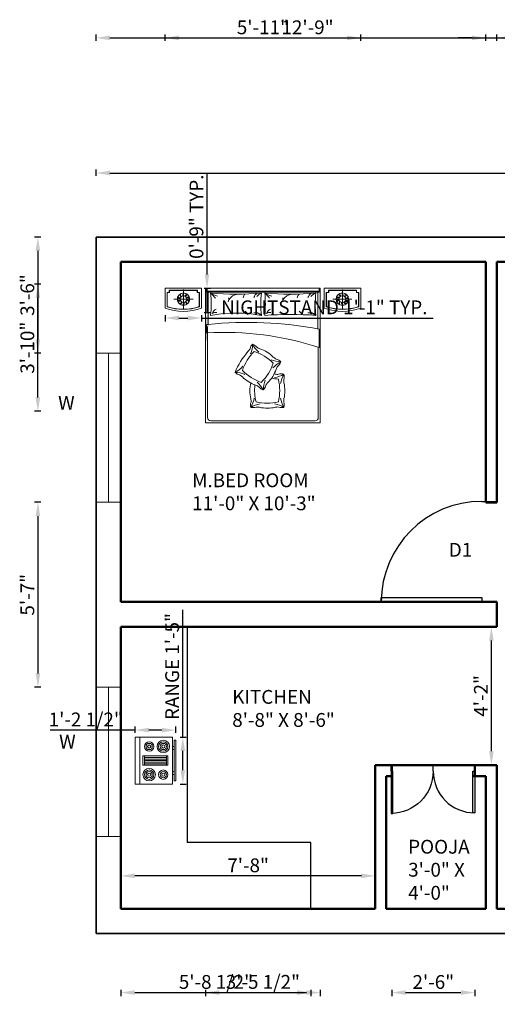
# Model space of a CAD drawing. Units: inches. Extents: x -26 to 423, y -281 to 96.
# Tile 1 of 3: x -26 to 147, y -264 to 92. Entities that reach past the tile are written whole.
import ezdxf

# ---------------------------------------------------------------- set-up
doc = ezdxf.new("R2010")
doc.units = ezdxf.units.IN
doc.header["$PDMODE"] = 35
doc.header["$PDSIZE"] = 5
for name, color, linetype, lineweight in [('A-ANNO-DIMS', 2, 'Continuous', 18), ('A-AREA-IDEN', 7, 'Continuous', 25), ('A-DOOR', 3, 'Continuous', 25), ('A-EQPM', 8, 'Continuous', 18), ('A-FLOR-CASE', 32, 'Continuous', 25), ('A-GLAZ', 4, 'Continuous', 18), ('A-WALL', 7, 'Continuous', 50), ('C-PROP', 7, 'Continuous', 35), ('furn', 28, 'Continuous', 18), ('txt', 167, 'Continuous', 18)]:
    doc.layers.add(name, color=color, linetype=linetype, lineweight=lineweight)
doc.styles.get("Standard").update_dxf_attribs({"font": 'arial.ttf'})
doc.dimstyles.new('ISO-25', dxfattribs={"dimtxt": 5, "dimasz": 5, "dimexe": 1.25, "dimexo": 0.625, "dimtad": 1, "dimlunit": 3, "dimtxsty": 'Standard', "dimcen": 2.5, "dimadec": 0, "dimazin": 0, "dimtfac": 1, "dimtmove": 0, "dimatfit": 3, "dimfxl": 1, "dimfxlon": 1, "dimarcsym": 0})

# ---------------------------------------------------------------- blocks, each defined once
blk = doc.blocks.new('*U2')
for p, q in [((0, 0), (0, -6)), ((40, 0), (40, -6))]:
    blk.add_line(p, q)
blk.add_lwpolyline([(0, 0), (0, 40), (1.75, 40), (1.75, 0)], close=True)
blk.add_arc((0, 0), 40, 0, 90)
blk = doc.blocks.new('Range-Oven - 30 in top')
for p, q in [((0, -3), (30, -3)), ((12, -6), (18, -6)), ((13, -20), (13, -6)), ((14, -6), (14, -20)), ((15, -20), (15, -6)), ((16, -6), (16, -20)), ((17, -20), (17, -6)), ((6, -24), (6, -25)), ((8, -25), (8, -24)), ((18, -20), (12, -20)), ((22, -25), (22, -24)), ((24, -24), (24, -25))]:
    blk.add_line(p, q)
for points in [[(0, -24), (0, 0), (30, 0), (30, -24)], [(12, -21), (12, -5), (18, -5), (18, -21)], [(2, -26), (2, -25), (28, -25), (28, -26)]]:
    blk.add_lwpolyline(points, close=True)
for centre, radius in [((6, -9), 4), ((6, -9), 3), ((24, -9), 3), ((6, -9), 2), ((6, -9), 1), ((24, -9), 2), ((24, -9), 1), ((6, -18), 3), ((6, -18), 2), ((6, -18), 1), ((24, -18), 4), ((24, -18), 3), ((24, -18), 2), ((24, -18), 1)]:
    blk.add_circle(centre, radius)
blk = doc.blocks.new('*D9')
at = {"layer": 'A-ANNO-DIMS', "color": 0, "lineweight": -2, "transparency": 16777216}
for p, q in [((144.67, -127.84), (145.92, -127.84)), ((144.67, -172.84), (144.67, -132.84)), ((145.67, -177.84), (143.42, -177.84))]:
    blk.add_line(p, q, dxfattribs=at)
at = {"layer": 'A-ANNO-DIMS', "color": 0, "transparency": 16777216}
for points in [[(143.84, -132.84), (145.51, -132.84), (144.67, -127.84)], [(143.84, -172.84), (145.51, -172.84), (144.67, -177.84)]]:
    blk.add_solid(points, dxfattribs=at)
at = {"layer": 'Defpoints', "color": 0, "transparency": 16777216}
for p in [(144.67, -127.84), (144.67, -127.84), (146.67, -177.84)]:
    blk.add_point(p, dxfattribs=at)
at = {"layer": 'A-ANNO-DIMS', "color": 0, "transparency": 16777216, "insert": (141.54, -152.84), "char_height": 5, "attachment_point": 5, "rotation": 90}
blk.add_mtext('4\'-2"', dxfattribs=at)
blk = doc.blocks.new('*D10')
at = {"layer": 'A-ANNO-DIMS', "color": 0, "lineweight": -2, "transparency": 16777216}
for p, q in [((10.67, -218.94), (10.67, -216.69)), ((102.67, -218.94), (102.67, -216.69)), ((97.67, -217.94), (15.67, -217.94))]:
    blk.add_line(p, q, dxfattribs=at)
at = {"layer": 'A-ANNO-DIMS', "color": 0, "transparency": 16777216}
for points in [[(15.67, -217.11), (15.67, -218.78), (10.67, -217.94)], [(97.67, -217.11), (97.67, -218.78), (102.67, -217.94)]]:
    blk.add_solid(points, dxfattribs=at)
at = {"layer": 'Defpoints', "color": 0, "transparency": 16777216}
for p in [(10.67, -217.94), (10.67, -226.07), (102.67, -229.84)]:
    blk.add_point(p, dxfattribs=at)
at = {"layer": 'A-ANNO-DIMS', "color": 0, "transparency": 16777216, "insert": (56.67, -214.77), "char_height": 5, "attachment_point": 5}
blk.add_mtext('7\'-8"', dxfattribs=at)
blk = doc.blocks.new('*D12')
at = {"layer": 'A-ANNO-DIMS', "color": 0, "lineweight": -2, "transparency": 16777216}
for p, q in [((1.67, 35.33), (1.67, 37.58)), ((6.67, 36.33), (392.67, 36.33)), ((397.67, 35.33), (397.67, 37.58))]:
    blk.add_line(p, q, dxfattribs=at)
at = {"layer": 'A-ANNO-DIMS', "color": 0, "transparency": 16777216}
for points in [[(6.67, 37.17), (6.67, 35.5), (1.67, 36.33)], [(392.67, 37.17), (392.67, 35.5), (397.67, 36.33)]]:
    blk.add_solid(points, dxfattribs=at)
at = {"layer": 'Defpoints', "color": 0, "transparency": 16777216}
for p in [(397.67, 36.33), (1.67, 13.16), (397.67, 13.16)]:
    blk.add_point(p, dxfattribs=at)
at = {"layer": 'A-ANNO-DIMS', "color": 0, "transparency": 16777216, "insert": (199.67, 39.51), "char_height": 5, "attachment_point": 5}
blk.add_mtext("33'", dxfattribs=at)
blk = doc.blocks.new('WINDOW-54IN')
blk.add_line((4.5, 54), (4.5, 0))
blk.add_lwpolyline([(0, 54), (9, 54), (9, 0), (0, 0)], close=True)
blk = doc.blocks.new('NIGHTSTAND-WIDE')
blk.add_lwpolyline([(0, 1.2), (0, 8.4), (13.2, 8.4), (13.2, 1.2, -0.181818)], format="xyb", close=True)
for points in [[(1.51, 7.68), (1.51, 6.89), (0.72, 6.89)], [(1.58, 7.68), (1.58, 6.82), (0.72, 6.82)], [(1.51, 7.68), (11.69, 7.68)], [(1.51, 7.61), (11.69, 7.61)], [(11.62, 7.68), (11.62, 6.82), (12.48, 6.82)], [(11.69, 7.68), (11.69, 6.89), (12.48, 6.89)]]:
    blk.add_lwpolyline(points)
for points in [[(12.48, 6.89), (12.48, 1.7, -0.167087), (0.72, 1.7), (0.72, 6.89)], [(12.41, 6.89), (12.41, 1.75, -0.165559), (0.79, 1.75), (0.79, 6.89)]]:
    blk.add_lwpolyline(points, format="xyb")
blk = doc.blocks.new('*D19')
at = {"layer": 'A-ANNO-DIMS', "color": 0, "lineweight": -2, "transparency": 16777216}
for p, q in [((26.61, -15.13), (26.61, -17.38)), ((31.61, -16.13), (34.82, -16.13)), ((39.82, -15.13), (39.82, -17.38)), ((39.82, -16.13), (123.64, -16.13))]:
    blk.add_line(p, q, dxfattribs=at)
at = {"layer": 'A-ANNO-DIMS', "color": 0, "transparency": 16777216}
for points in [[(31.61, -15.29), (31.61, -16.96), (26.61, -16.13)], [(34.82, -15.29), (34.82, -16.96), (39.82, -16.13)]]:
    blk.add_solid(points, dxfattribs=at)
at = {"layer": 'Defpoints', "color": 0, "transparency": 16777216}
for p in [(26.61, -14.14), (39.82, -14.14), (39.82, -16.13)]:
    blk.add_point(p, dxfattribs=at)
at = {"layer": 'A-ANNO-DIMS', "color": 0, "transparency": 16777216, "insert": (84.23, -12.91), "char_height": 5, "attachment_point": 5}
blk.add_mtext('NIGHTSTAND 1\'-1" TYP.', dxfattribs=at)
blk = doc.blocks.new('*D20')
at = {"layer": 'A-ANNO-DIMS', "color": 0, "lineweight": -2, "transparency": 16777216}
for p, q in [((41.8, -0.34), (41.8, 36.39)), ((40.8, -5.34), (43.05, -5.34)), ((41.8, -14.14), (41.8, -5.34)), ((40.8, -14.14), (43.05, -14.14)), ((41.8, -19.14), (41.8, -24.14))]:
    blk.add_line(p, q, dxfattribs=at)
at = {"layer": 'A-ANNO-DIMS', "color": 0, "transparency": 16777216}
for points in [[(40.96, -0.34), (42.63, -0.34), (41.8, -5.34)], [(40.96, -19.14), (42.63, -19.14), (41.8, -14.14)]]:
    blk.add_solid(points, dxfattribs=at)
at = {"layer": 'Defpoints', "color": 0, "transparency": 16777216}
for p in [(39.82, -5.34), (41.8, -5.34), (39.82, -14.14)]:
    blk.add_point(p, dxfattribs=at)
at = {"layer": 'A-ANNO-DIMS', "color": 0, "transparency": 16777216, "insert": (38.62, 20.52), "char_height": 5, "attachment_point": 5, "rotation": 90}
blk.add_mtext('0\'-9" TYP.', dxfattribs=at)
blk = doc.blocks.new('*D29')
at = {"layer": 'A-ANNO-DIMS', "color": 0, "lineweight": -2, "transparency": 16777216}
for p, q in [((33.05, -167.76), (33.05, -121.69)), ((32.05, -167.76), (34.3, -167.76)), ((33.05, -179.73), (33.05, -172.76)), ((32.05, -184.73), (34.3, -184.73))]:
    blk.add_line(p, q, dxfattribs=at)
at = {"layer": 'A-ANNO-DIMS', "color": 0, "transparency": 16777216}
for points in [[(32.21, -172.76), (33.88, -172.76), (33.05, -167.76)], [(32.21, -179.73), (33.88, -179.73), (33.05, -184.73)]]:
    blk.add_solid(points, dxfattribs=at)
at = {"layer": 'Defpoints', "color": 0, "transparency": 16777216}
for p in [(30.5, -167.76), (33.05, -167.76), (30.5, -184.73)]:
    blk.add_point(p, dxfattribs=at)
at = {"layer": 'A-ANNO-DIMS', "color": 0, "transparency": 16777216, "insert": (29.84, -142.22), "char_height": 5, "attachment_point": 5, "rotation": 90}
blk.add_mtext('RANGE 1\'-5"', dxfattribs=at)
blk = doc.blocks.new('*D30')
at = {"layer": 'A-ANNO-DIMS', "color": 0, "lineweight": -2, "transparency": 16777216}
for p, q in [((15.79, -165.21), (-14.93, -165.21)), ((15.79, -166.21), (15.79, -163.96)), ((25.5, -165.21), (20.79, -165.21)), ((30.5, -166.21), (30.5, -163.96))]:
    blk.add_line(p, q, dxfattribs=at)
at = {"layer": 'A-ANNO-DIMS', "color": 0, "transparency": 16777216}
for points in [[(20.79, -164.38), (20.79, -166.04), (15.79, -165.21)], [(25.5, -164.38), (25.5, -166.04), (30.5, -165.21)]]:
    blk.add_solid(points, dxfattribs=at)
at = {"layer": 'Defpoints', "color": 0, "transparency": 16777216}
for p in [(15.79, -165.21), (15.79, -167.76), (30.5, -167.76)]:
    blk.add_point(p, dxfattribs=at)
at = {"layer": 'A-ANNO-DIMS', "color": 0, "transparency": 16777216, "insert": (-2.07, -162), "char_height": 5, "attachment_point": 5}
blk.add_mtext('1\'-2 1/2"', dxfattribs=at)
blk = doc.blocks.new('*D31')
at = {"layer": 'A-ANNO-DIMS', "color": 0, "lineweight": -2, "transparency": 16777216}
for p, q in [((-18.38, 13.16), (-20.63, 13.16)), ((-19.38, 8.16), (-19.38, -23.8)), ((-18.38, -28.8), (-20.63, -28.8))]:
    blk.add_line(p, q, dxfattribs=at)
at = {"layer": 'A-ANNO-DIMS', "color": 0, "transparency": 16777216}
for points in [[(-20.22, 8.16), (-18.55, 8.16), (-19.38, 13.16)], [(-20.22, -23.8), (-18.55, -23.8), (-19.38, -28.8)]]:
    blk.add_solid(points, dxfattribs=at)
at = {"layer": 'Defpoints', "color": 0, "transparency": 16777216}
for p in [(1.67, 13.16), (-19.38, -28.8), (1.67, -28.8)]:
    blk.add_point(p, dxfattribs=at)
at = {"layer": 'A-ANNO-DIMS', "color": 0, "transparency": 16777216, "insert": (-22.56, -7.82), "char_height": 5, "attachment_point": 5, "rotation": 90}
blk.add_mtext('3\'-6"', dxfattribs=at)
blk = doc.blocks.new('*D32')
at = {"layer": 'A-ANNO-DIMS', "color": 0, "lineweight": -2, "transparency": 16777216}
for p, q in [((-18.38, -82.8), (-20.63, -82.8)), ((-19.38, -87.8), (-19.38, -144.68)), ((-18.38, -149.68), (-20.63, -149.68))]:
    blk.add_line(p, q, dxfattribs=at)
at = {"layer": 'A-ANNO-DIMS', "color": 0, "transparency": 16777216}
for points in [[(-20.22, -87.8), (-18.55, -87.8), (-19.38, -82.8)], [(-20.22, -144.68), (-18.55, -144.68), (-19.38, -149.68)]]:
    blk.add_solid(points, dxfattribs=at)
at = {"layer": 'Defpoints', "color": 0, "transparency": 16777216}
for p in [(1.67, -82.8), (-19.38, -149.68), (1.67, -149.68)]:
    blk.add_point(p, dxfattribs=at)
at = {"layer": 'A-ANNO-DIMS', "color": 0, "transparency": 16777216, "insert": (-22.55, -116.24), "char_height": 5, "attachment_point": 5, "rotation": 90}
blk.add_mtext('5\'-7"', dxfattribs=at)
blk = doc.blocks.new('*D33')
at = {"layer": 'A-ANNO-DIMS', "color": 0, "lineweight": -2, "transparency": 16777216}
for p, q in [((1.67, 84.21), (1.67, 86.46)), ((154.67, 84.21), (154.67, 86.46)), ((6.67, 85.21), (149.67, 85.21))]:
    blk.add_line(p, q, dxfattribs=at)
at = {"layer": 'A-ANNO-DIMS', "color": 0, "transparency": 16777216}
for points in [[(6.67, 86.05), (6.67, 84.38), (1.67, 85.21)], [(149.67, 86.05), (149.67, 84.38), (154.67, 85.21)]]:
    blk.add_solid(points, dxfattribs=at)
at = {"layer": 'Defpoints', "color": 0, "transparency": 16777216}
for p in [(154.67, 85.21), (1.67, 13.16), (154.67, 13.16)]:
    blk.add_point(p, dxfattribs=at)
at = {"layer": 'A-ANNO-DIMS', "color": 0, "transparency": 16777216, "insert": (78.17, 88.39), "char_height": 5, "attachment_point": 5}
blk.add_mtext('12\'-9"', dxfattribs=at)
blk = doc.blocks.new('*D40')
at = {"layer": 'A-ANNO-DIMS', "color": 0, "lineweight": -2, "transparency": 16777216}
for p, q in [((108.67, -259.17), (108.67, -261.42)), ((138.67, -259.17), (138.67, -261.42)), ((113.67, -260.17), (133.67, -260.17))]:
    blk.add_line(p, q, dxfattribs=at)
at = {"layer": 'A-ANNO-DIMS', "color": 0, "transparency": 16777216}
for points in [[(113.67, -259.33), (113.67, -261), (108.67, -260.17)], [(133.67, -259.33), (133.67, -261), (138.67, -260.17)]]:
    blk.add_solid(points, dxfattribs=at)
at = {"layer": 'Defpoints', "color": 0, "transparency": 16777216}
for p in [(108.67, -177.84), (138.67, -177.84), (138.67, -260.17)]:
    blk.add_point(p, dxfattribs=at)
at = {"layer": 'A-ANNO-DIMS', "color": 0, "transparency": 16777216, "insert": (123.67, -256.99), "char_height": 5, "attachment_point": 5}
blk.add_mtext('2\'-6"', dxfattribs=at)
blk = doc.blocks.new('*D46')
at = {"layer": 'A-ANNO-DIMS', "color": 0, "lineweight": -2, "transparency": 16777216}
for p, q in [((41.26, -259.17), (41.26, -261.42)), ((82.79, -259.17), (82.79, -261.42)), ((46.26, -260.17), (77.79, -260.17))]:
    blk.add_line(p, q, dxfattribs=at)
at = {"layer": 'A-ANNO-DIMS', "color": 0, "transparency": 16777216}
for points in [[(46.26, -259.33), (46.26, -261), (41.26, -260.17)], [(77.79, -259.33), (77.79, -261), (82.79, -260.17)]]:
    blk.add_solid(points, dxfattribs=at)
at = {"layer": 'Defpoints', "color": 0, "transparency": 16777216}
for p in [(41.26, -54.07), (82.79, -54.07), (82.79, -260.17)]:
    blk.add_point(p, dxfattribs=at)
at = {"layer": 'A-ANNO-DIMS', "color": 0, "transparency": 16777216, "insert": (62.02, -256.95), "char_height": 5, "attachment_point": 5}
blk.add_mtext('3\'-5 1/2"', dxfattribs=at)
blk = doc.blocks.new('*D47')
at = {"layer": 'A-ANNO-DIMS', "color": 0, "lineweight": -2, "transparency": 16777216}
for p, q in [((417.73, -5.34), (419.98, -5.34)), ((418.73, -49.07), (418.73, -10.34)), ((417.73, -54.07), (419.98, -54.07))]:
    blk.add_line(p, q, dxfattribs=at)
at = {"layer": 'A-ANNO-DIMS', "color": 0, "transparency": 16777216}
for points in [[(417.89, -10.34), (419.56, -10.34), (418.73, -5.34)], [(417.89, -49.07), (419.56, -49.07), (418.73, -54.07)]]:
    blk.add_solid(points, dxfattribs=at)
at = {"layer": 'Defpoints', "color": 0, "transparency": 16777216}
for p in [(82.79, -5.34), (418.73, -5.34), (82.79, -54.07)]:
    blk.add_point(p, dxfattribs=at)
at = {"layer": 'A-ANNO-DIMS', "color": 0, "transparency": 16777216, "insert": (415.52, -29.71), "char_height": 5, "attachment_point": 5, "rotation": 90}
blk.add_mtext('4\'-0 1/2"', dxfattribs=at)
blk = doc.blocks.new('*D50')
at = {"layer": 'A-ANNO-DIMS', "color": 0, "lineweight": -2, "transparency": 16777216}
for p, q in [((26.61, 84.21), (26.61, 86.46)), ((97.44, 84.21), (97.44, 86.46)), ((31.61, 85.21), (92.44, 85.21))]:
    blk.add_line(p, q, dxfattribs=at)
at = {"layer": 'A-ANNO-DIMS', "color": 0, "transparency": 16777216}
for points in [[(31.61, 86.05), (31.61, 84.38), (26.61, 85.21)], [(92.44, 86.05), (92.44, 84.38), (97.44, 85.21)]]:
    blk.add_solid(points, dxfattribs=at)
at = {"layer": 'Defpoints', "color": 0, "transparency": 16777216}
for p in [(97.44, 85.21), (26.61, -5.34), (97.44, -5.34)]:
    blk.add_point(p, dxfattribs=at)
at = {"layer": 'A-ANNO-DIMS', "color": 0, "transparency": 16777216, "insert": (62.02, 88.39), "char_height": 5, "attachment_point": 5}
blk.add_mtext('5\'-11"', dxfattribs=at)
blk = doc.blocks.new('*D51')
at = {"layer": 'A-ANNO-DIMS', "color": 0, "lineweight": -2, "transparency": 16777216}
for p, q in [((-18.38, -3.86), (-20.63, -3.86)), ((-19.38, -44.88), (-19.38, -8.86)), ((-18.38, -49.88), (-20.63, -49.88))]:
    blk.add_line(p, q, dxfattribs=at)
at = {"layer": 'A-ANNO-DIMS', "color": 0, "transparency": 16777216}
for points in [[(-20.22, -8.86), (-18.55, -8.86), (-19.38, -3.86)], [(-20.22, -44.88), (-18.55, -44.88), (-19.38, -49.88)]]:
    blk.add_solid(points, dxfattribs=at)
at = {"layer": 'Defpoints', "color": 0, "transparency": 16777216}
for p in [(-19.38, -3.86), (222.74, -3.86), (222.74, -49.88)]:
    blk.add_point(p, dxfattribs=at)
at = {"layer": 'A-ANNO-DIMS', "color": 0, "transparency": 16777216, "insert": (-22.56, -26.87), "char_height": 5, "attachment_point": 5, "rotation": 90}
blk.add_mtext('3\'-10"', dxfattribs=at)
blk = doc.blocks.new('*D54')
at = {"layer": 'A-ANNO-DIMS', "color": 0, "lineweight": -2, "transparency": 16777216}
for p, q in [((142.67, 84.21), (142.67, 86.46)), ((146.67, 84.21), (146.67, 86.46)), ((137.67, 85.21), (132.67, 85.21)), ((142.67, 85.21), (146.67, 85.21)), ((151.67, 85.21), (171.21, 85.21))]:
    blk.add_line(p, q, dxfattribs=at)
at = {"layer": 'A-ANNO-DIMS', "color": 0, "transparency": 16777216}
for points in [[(137.67, 86.05), (137.67, 84.38), (142.67, 85.21)], [(151.67, 86.05), (151.67, 84.38), (146.67, 85.21)]]:
    blk.add_solid(points, dxfattribs=at)
at = {"layer": 'Defpoints', "color": 0, "transparency": 16777216}
for p in [(146.67, 85.21), (142.67, 4.16), (146.67, 4.16)]:
    blk.add_point(p, dxfattribs=at)
at = {"layer": 'A-ANNO-DIMS', "color": 0, "transparency": 16777216, "insert": (163.94, 88.39), "char_height": 5, "attachment_point": 5}
blk.add_mtext('0\'-4"', dxfattribs=at)
blk = doc.blocks.new('*D55')
at = {"layer": 'A-ANNO-DIMS', "color": 0, "lineweight": -2, "transparency": 16777216}
for p, q in [((417.73, -205.84), (419.98, -205.84)), ((418.73, -210.84), (418.73, -224.84)), ((417.73, -229.84), (419.98, -229.84))]:
    blk.add_line(p, q, dxfattribs=at)
at = {"layer": 'A-ANNO-DIMS', "color": 0, "transparency": 16777216}
for points in [[(417.89, -210.84), (419.56, -210.84), (418.73, -205.84)], [(417.89, -224.84), (419.56, -224.84), (418.73, -229.84)]]:
    blk.add_solid(points, dxfattribs=at)
at = {"layer": 'Defpoints', "color": 0, "transparency": 16777216}
for p in [(79.39, -205.84), (79.39, -229.84), (418.73, -229.84)]:
    blk.add_point(p, dxfattribs=at)
at = {"layer": 'A-ANNO-DIMS', "color": 0, "transparency": 16777216, "insert": (415.55, -217.84), "char_height": 5, "attachment_point": 5, "rotation": 90}
blk.add_mtext('2\'-0"', dxfattribs=at)
blk = doc.blocks.new('*D56')
at = {"layer": 'A-ANNO-DIMS', "color": 0, "lineweight": -2, "transparency": 16777216}
for p, q in [((10.67, -259.17), (10.67, -261.42)), ((79.39, -259.17), (79.39, -261.42)), ((15.67, -260.17), (74.39, -260.17))]:
    blk.add_line(p, q, dxfattribs=at)
at = {"layer": 'A-ANNO-DIMS', "color": 0, "transparency": 16777216}
for points in [[(15.67, -259.33), (15.67, -261), (10.67, -260.17)], [(74.39, -259.33), (74.39, -261), (79.39, -260.17)]]:
    blk.add_solid(points, dxfattribs=at)
at = {"layer": 'Defpoints', "color": 0, "transparency": 16777216}
for p in [(10.67, -229.84), (79.39, -229.84), (79.39, -260.17)]:
    blk.add_point(p, dxfattribs=at)
at = {"layer": 'A-ANNO-DIMS', "color": 0, "transparency": 16777216, "insert": (45.03, -256.96), "char_height": 5, "attachment_point": 5}
blk.add_mtext('5\'-8 1/2"', dxfattribs=at)

msp = doc.modelspace()

# ---------------------------------------------------------------- linework, layer by layer
at = {"layer": 'A-FLOR-CASE'}
for p, q in [((34.673, -127.842), (34.673, -205.842)), ((79.395, -205.842), (34.673, -205.842)), ((79.395, -229.842), (79.395, -205.842))]:
    msp.add_line(p, q, dxfattribs=at)
at = {"layer": 'A-WALL'}
for p, q in [((10.673, 4.158), (142.673, 4.158)), ((10.673, -118.842), (10.673, 4.158)), ((142.673, -82.842), (142.673, 4.158)), ((146.673, 4.158), (198.673, 4.158)), ((146.673, -82.842), (146.673, 4.158)), ((146.673, -82.842), (142.673, -82.842)), ((10.673, -118.842), (142.673, -118.842)), ((142.673, -118.842), (146.673, -118.842)), ((146.673, -127.842), (146.673, -118.842)), ((10.673, -229.842), (10.673, -127.842)), ((10.673, -127.842), (142.673, -127.842)), ((142.673, -127.842), (146.673, -127.842)), ((102.673, -229.842), (102.673, -177.842)), ((106.673, -177.842), (102.673, -177.842)), ((106.673, -177.842), (142.673, -177.842)), ((108.673, -177.842), (108.673, -181.842)), ((138.673, -177.842), (138.673, -181.842)), ((142.673, -177.842), (146.673, -177.842)), ((146.673, -229.842), (146.673, -177.842)), ((106.673, -229.842), (106.673, -181.842)), ((106.673, -181.842), (109.075, -181.842)), ((138.014, -181.842), (142.673, -181.842)), ((142.673, -229.842), (142.673, -181.842)), ((102.673, -229.842), (10.673, -229.842)), ((142.673, -229.842), (106.673, -229.842)), ((142.673, -229.842), (142.673, -229.842)), ((198.673, -229.842), (146.673, -229.842))]:
    msp.add_line(p, q, dxfattribs=at)
at = {"layer": 'C-PROP'}
for p, q in [((1.673, 13.158), (397.673, 13.158)), ((1.673, -238.842), (1.673, 13.158)), ((397.673, -238.842), (1.673, -238.842))]:
    msp.add_line(p, q, dxfattribs=at)
at = {"layer": 'furn'}
for p, q in [((33.282, -12.779), (33.282, -5.855)), ((41.977, -6.822), (82.071, -6.822)), ((42.182, -6.464), (42.182, -18.456)), ((81.841, -6.464), (81.841, -20.015)), ((90.765, -12.78), (90.765, -5.856)), ((29.82, -9.317), (36.744, -9.317)), ((94.228, -9.318), (87.303, -9.318))]:
    msp.add_line(p, q, dxfattribs=at)
for points in [[(41.257, -5.338), (41.257, -54.075), (82.791, -54.075), (82.791, -5.338)], [(82.403, -5.338), (82.403, -6.464), (41.497, -6.464), (41.497, -5.338), (82.791, -5.338)]]:
    msp.add_lwpolyline(points, dxfattribs=at)
for points in [[(43.098, -15.175, 0.0585956), (43.098, -7.152, 0.0368889), (61.482, -7.152, 0.052163), (61.482, -15.175, 0.0931113)], [(62.677, -15.175, 0.0585956), (62.677, -7.152, 0.0366479), (81.181, -7.152, 0.052163), (81.181, -15.175, 0.0369674)], [(41.62, -18.456), (42.182, -18.456, -0.0729439), (82.403, -20.131), (82.403, -26.79, 0.0925678), (41.62, -21.51)]]:
    msp.add_lwpolyline(points, format="xyb", close=True, dxfattribs=at)
for points in [[(41.977, -21.489), (41.977, -52.154, 0.4142136), (43.177, -53.355), (80.87, -53.355, 0.4142136), (82.071, -52.154), (82.071, -26.672)], [(54.592, -35.146, 0.1110065), (61.45, -39.41, 0.1195491), (65.773, -32.472, 0.1078134), (58.936, -28.189)], [(58.899, -28.198, 0.1218652), (54.593, -35.145, 0.1218652)], [(57.567, -29.137, 0.0912961), (58.296, -25.619, 0.0912961), (60.51, -28.448, 0.0912961)], [(62.136, -42.156, 0.1594612), (63.066, -40.507, -0.0762829), (63.804, -39.48, 0.1150751), (66.817, -34.643, -0.0762829), (67.414, -33.529, 0.1594612), (68.484, -31.968)], [(64.97, -31.227, 0.0912961), (68.484, -31.968, 0.0912961), (65.649, -34.172, 0.0912961)], [(55.463, -36.549, 0.0912961), (51.948, -35.808, 0.0912961), (54.784, -33.603, 0.0912961)], [(59.531, -46.489, 0.1110065), (67.606, -46.481, 0.1195491), (67.606, -38.306, 0.0332124), (65.123, -37.929)], [(62.866, -38.639, 0.0912961), (62.136, -42.156, 0.0912961), (59.922, -39.327)], [(66.266, -37.675, 0.0912961), (69.641, -36.445, 0.0912961), (68.4, -39.816, 0.0912961)], [(69.641, -48.449, 0.1594612), (69.558, -46.558, -0.0762829), (69.641, -45.296, 0.1150751), (69.641, -39.598, -0.0762829), (69.558, -38.336, 0.1594612), (69.641, -36.445)], [(61.011, -47.219, 0.0912961), (57.636, -48.449, 0.0912961), (58.877, -45.078, 0.0912961)], [(68.4, -45.078, 0.0912961), (69.641, -48.449, 0.0912961), (66.266, -47.219)]]:
    msp.add_lwpolyline(points, format="xyb", dxfattribs=at)
for centre, radius in [((33.282, -9.317), 2.262), ((90.765, -9.318), 2.262), ((33.282, -9.317), 1.225), ((90.765, -9.318), 1.225)]:
    msp.add_circle(centre, radius, dxfattribs=at)
for centre, radius, start, end in [((34.44, -8.065), 1.453, 136.17003, 182.48975), ((34.307, -8.007), 1.108, 124.30017, 184.53802), ((41.977, -6.102), 0.72, 180, 270), ((82.071, -6.102), 0.72, 270, 0), ((89.741, -8.008), 1.108, 355.46198, 55.69983), ((89.608, -8.065), 1.453, 357.51025, 43.82997), ((31.719, -8.748), 1.108, 232.30017, 292.53802), ((31.733, -8.603), 1.453, 244.17003, 290.48975), ((32.448, -7.829), 1.453, 208.17003, 254.48975), ((32.352, -7.938), 1.108, 196.30017, 256.53802), ((31.683, -9.775), 1.108, 268.30017, 328.53802), ((31.609, -9.65), 1.453, 280.17003, 326.48975), ((33.482, -7.623), 1.453, 172.17003, 218.48975), ((33.341, -7.655), 1.108, 160.30017, 220.53802), ((32.258, -10.628), 1.108, 304.30017, 4.53802), ((32.124, -10.57), 1.453, 316.17003, 2.48975), ((34.955, -8.984), 1.453, 100.17003, 146.48975), ((34.881, -8.859), 1.108, 88.30017, 148.53802), ((33.224, -10.98), 1.108, 340.30017, 40.53802), ((33.082, -11.011), 1.453, 352.17003, 38.48975), ((34.831, -10.031), 1.453, 64.17003, 110.48975), ((34.845, -9.887), 1.108, 52.30017, 112.53802), ((34.212, -10.697), 1.108, 16.30017, 76.53802), ((34.116, -10.806), 1.453, 28.17003, 74.48975), ((47.365, -0.445), 7.95, 237.53791, 257.5233), ((37.083, -14.655), 9.617, 36.49353, 51.27919), ((47.687, -9.434), 1.994, 335.89274, 16.11919), ((53.463, -11.91), 4.45, 96.68493, 148.3182), ((57.963, -9.379), 3.121, 141.81741, 169.89867), ((61.91, -9.822), 3.358, 130.53543, 160.35581), ((64.005, -12.652), 6.051, 114.64565, 134.15848), ((56.661, -14.655), 9.617, 36.49353, 51.27919), ((66.944, -0.445), 7.95, 237.53791, 257.5233), ((67.266, -9.434), 1.994, 335.89274, 16.11919), ((73.042, -11.91), 4.45, 96.68493, 148.3182), ((77.542, -9.379), 3.121, 141.81741, 169.89867), ((81.489, -9.822), 3.358, 130.53543, 160.35581), ((83.584, -12.652), 6.051, 114.64565, 134.15848), ((89.203, -9.888), 1.108, 67.46198, 127.69983), ((89.216, -10.032), 1.453, 69.51025, 115.82997), ((89.932, -10.806), 1.453, 105.51025, 151.82997), ((89.836, -10.697), 1.108, 103.46198, 163.69983), ((89.166, -8.86), 1.108, 31.46198, 91.69983), ((89.092, -8.985), 1.453, 33.51025, 79.82997), ((90.966, -11.012), 1.453, 141.51025, 187.82997), ((90.824, -10.981), 1.108, 139.46198, 199.69983), ((91.923, -10.571), 1.453, 177.51025, 223.82997), ((91.79, -10.629), 1.108, 175.46198, 235.69983), ((92.439, -9.651), 1.453, 213.51025, 259.82997), ((92.365, -9.776), 1.108, 211.46198, 271.69983), ((90.707, -7.656), 1.108, 319.46198, 19.69983), ((90.73, -7.562), 1.453, 321.51025, 7.82997), ((92.479, -8.542), 1.453, 249.51025, 295.82997), ((92.493, -8.686), 1.108, 247.46198, 307.69983), ((91.86, -7.876), 1.108, 283.46198, 343.69983), ((91.764, -7.768), 1.453, 285.51025, 331.82997), ((46.258, -15.36), 2.668, 114.2916, 160.9896), ((44.874, -15.918), 1.825, 76.48229, 128.55627), ((48.509, -20.756), 10.023, 36.20852, 45.08491), ((55.923, -14.835), 0.673, 353.75428, 77.21866), ((59.138, -17.471), 3.281, 44.40604, 96.83423), ((59.751, -16.327), 2.079, 33.63488, 90.84559), ((65.837, -15.36), 2.668, 114.2916, 160.9896), ((64.452, -15.918), 1.825, 76.48229, 128.55627), ((68.087, -20.756), 10.023, 36.20852, 45.08491), ((75.502, -14.835), 0.673, 353.75428, 77.21866), ((78.717, -17.471), 3.281, 44.40604, 96.83423), ((79.33, -16.327), 2.079, 33.63488, 90.84559), ((76.283, -45.756), 26.29, 138.38179, 157.76439), ((53.652, -25.378), 4.168, 315.58539, 333.03435), ((60.351, -27.864), 3.043, 132.46578, 168.70648), ((57.492, -28.443), 2.936, 37.29372, 74.09733), ((62.319, -23.322), 4.168, 233.29829, 250.74724), ((56.941, -39.145), 12.544, 45.13065, 71.38844), ((68.698, -27.268), 4.168, 225.77185, 243.2208), ((66.315, -33.754), 2.81, 39.47264, 79.6505), ((54.186, -33.746), 3.043, 222.65224, 258.89294), ((51.722, -40.453), 4.168, 45.77185, 63.2208), ((63.479, -28.576), 12.544, 225.13065, 251.38844), ((63.639, -48.641), 12.544, 77.05756, 78.7033), ((67.337, -32.344), 4.168, 257.69876, 275.14771), ((68.744, -39.108), 2.81, 71.39955, 111.57741), ((69.853, -42.447), 12.544, 166.87111, 193.12889), ((76.041, -42.363), 17.018, 173.19556, 194.02838), ((58.101, -44.399), 4.168, 53.29829, 70.74724), ((63.307, -38.877), 3.482, 218.77541, 250.35713), ((53.567, -46.198), 4.168, 355.03874, 12.4877), ((60.567, -47.63), 3.043, 159.36661, 195.60731), ((58.446, -45.516), 3.043, 254.57915, 290.81985), ((59.901, -52.511), 4.168, 77.69876, 95.14771), ((63.599, -36.213), 12.544, 257.05756, 283.31535), ((67.402, -52.487), 4.168, 85.2252, 102.67415), ((68.9, -45.047), 3.482, 250.70232, 282.28404)]:
    msp.add_arc(centre, radius, start, end, dxfattribs=at)

# ---------------------------------------------------------------- block references
at = {"layer": 'A-DOOR'}
for p, xscale, yscale, zscale, rotation in [((141.214, -118.842), 0.9097136077923842, 0.9097136077923842, 0.9097136077923842, 90), ((108.409, -180.124), -0.3802872973524125, 0.3802872973524125, 0.3802872973524125, 180), ((138.673, -180.1), 0.3762966301077644, 0.3762966301077644, 0.3762966301077644, 180)]:
    msp.add_blockref('*U2', p, dxfattribs=dict(at, xscale=xscale, yscale=yscale, zscale=zscale, rotation=rotation))
at = {"layer": 'A-EQPM', "xscale": 0.5656854343773281, "yscale": 0.5656854343773281, "zscale": 0.5656854343773281, "rotation": 90}
msp.add_blockref('Range-Oven - 30 in top', (15.794, -184.727), dxfattribs=at)
at = {"layer": 'A-GLAZ'}
for p in [(1.673, -82.796), (1.673, -203.681)]:
    msp.add_blockref('WINDOW-54IN', p, dxfattribs=at)
at = {"layer": 'furn'}
msp.add_blockref('NIGHTSTAND-WIDE', (26.612, -13.744), dxfattribs=at)
at = {"layer": 'furn', "extrusion": (0, 0, -1), "zscale": -1, "rotation": 6.5579598125e-06}
msp.add_blockref('NIGHTSTAND-WIDE', (-97.436, -13.741), dxfattribs=at)

# ---------------------------------------------------------------- texts
at = {"layer": 'A-AREA-IDEN', "char_height": 5, "attachment_point": 1}
for s, width, insert in [('M.BED ROOM\\P11\'-0" X 10\'-3"', 45.91548, (36.421, -72.331)), ('KITCHEN\\P8\'-8" X 8\'-6"', 70.00456, (50.931, -150.701)), ('POOJA\\P3\'-0" X 4\'-0"', 24.38641, (114.584, -204.904))]:
    msp.add_mtext_dynamic_manual_height_columns(s, width=width, gutter_width=12.5, heights=[0], dxfattribs=dict(at, insert=insert))
at = {"layer": 'txt', "char_height": 5, "attachment_point": 1}
for s, width, insert in [('W', 8.40091, (-12.07, -44.281)), ('D1', 13.13388, (129.278, -97.484)), ('W', 8.58515, (-11.702, -166.904))]:
    msp.add_mtext_dynamic_manual_height_columns(s, width=width, gutter_width=12.5, heights=[0], dxfattribs=dict(at, insert=insert))

# ---------------------------------------------------------------- dimensions: what is measured, and where the dimension line sits
at = {"layer": 'A-ANNO-DIMS'}
for base, p1, p2, override, picture, middle in [((154.673, 85.213), (1.673, 13.158), (154.673, 13.158), {"dimdec": 1, "dimlfac": 1, "dimrnd": 0, "dimzin": 1, "dimdsep": 46, "dimlunit": 4, "dimfrac": 2}, '*D33', (78.173, 88.391)), ((97.436, 85.213), (26.612, -5.342), (97.436, -5.339), {"dimdec": 1, "dimlfac": 1, "dimrnd": 0, "dimzin": 1, "dimdsep": 46, "dimlunit": 4, "dimfrac": 2}, '*D50', (62.024, 88.391)), ((146.673, 85.213), (142.673, 4.158), (146.673, 4.158), {"dimdec": 1, "dimlfac": 1, "dimrnd": 0, "dimzin": 1, "dimdsep": 46, "dimlunit": 4, "dimfrac": 2}, '*D54', (163.943, 88.391)), ((397.673, 36.334), (1.673, 13.158), (397.673, 13.158), {"dimclrd": 0, "dimclre": 0, "dimclrt": 0}, '*D12', (199.673, 39.514)), ((82.791, -260.167), (41.257, -54.075), (82.791, -54.075), {"dimdec": 1, "dimlfac": 1, "dimrnd": 0, "dimzin": 1, "dimdsep": 46, "dimlunit": 4, "dimfrac": 2}, '*D46', (62.024, -256.955)), ((138.673, -260.167), (108.673, -177.842), (138.673, -177.842), {"dimdec": 1, "dimlfac": 1, "dimrnd": 0, "dimzin": 1, "dimdsep": 46, "dimlunit": 4, "dimfrac": 2}, '*D40', (123.673, -256.989)), ((10.673, -217.944), (102.673, -229.842), (10.673, -226.067), {"dimclrd": 0, "dimclre": 0, "dimclrt": 0}, '*D10', (56.673, -214.766)), ((79.395, -260.167), (10.673, -229.842), (79.395, -229.842), {"dimdec": 1, "dimlfac": 1, "dimrnd": 0, "dimzin": 1, "dimdsep": 46, "dimlunit": 4, "dimfrac": 2}, '*D56', (45.034, -256.956))]:
    dim = msp.add_linear_dim(base=base, p1=p1, p2=p2, dimstyle='ISO-25', override=override, dxfattribs=at)
    dim.commit()
    dim.dimension.update_dxf_attribs({"geometry": picture, "text_midpoint": middle})
for base, p1, p2, text, picture, middle in [((41.797, -5.342), (39.816, -14.145), (39.816, -5.342), '<> TYP.', '*D20', (38.619, 20.522)), ((33.048, -167.756), (30.502, -184.727), (30.502, -167.756), 'RANGE <>', '*D29', (29.837, -142.225))]:
    dim = msp.add_linear_dim(base=base, p1=p1, p2=p2, angle=90, text=text, dimstyle='ISO-25', override={"dimdec": 1, "dimlfac": 1, "dimrnd": 0, "dimzin": 1, "dimdsep": 46, "dimlunit": 4, "dimfrac": 2}, dxfattribs=at)
    dim.commit()
    dim.dimension.update_dxf_attribs({"geometry": picture, "text_midpoint": middle})
for base, p1, p2, angle, override, picture, middle in [((-19.382, -28.796), (1.673, 13.158), (1.673, -28.796), 90, {"dimdec": 1, "dimlfac": 1, "dimrnd": 0, "dimzin": 1, "dimdsep": 46, "dimlunit": 4, "dimfrac": 2}, '*D31', (-22.562, -7.819)), ((-19.382, -3.864), (222.744, -49.879), (222.742, -3.864), 90, {"dimdec": 1, "dimlfac": 1, "dimrnd": 0, "dimzin": 1, "dimdsep": 46, "dimlunit": 4, "dimfrac": 2}, '*D51', (-22.562, -26.871)), ((418.728, -5.338), (82.791, -54.075), (82.791, -5.338), 90, {"dimdec": 1, "dimlfac": 1, "dimrnd": 0, "dimzin": 1, "dimdsep": 46, "dimlunit": 4, "dimfrac": 2}, '*D47', (415.517, -29.707)), ((-19.382, -149.681), (1.673, -82.796), (1.673, -149.681), 90, {"dimdec": 1, "dimlfac": 1, "dimrnd": 0, "dimzin": 1, "dimdsep": 46, "dimlunit": 4, "dimfrac": 2}, '*D32', (-22.55, -116.238)), ((144.673, -127.842), (146.673, -177.842), (144.673, -127.842), 90, {"dimclrd": 0, "dimclre": 0, "dimclrt": 0}, '*D9', (141.537, -152.842)), ((15.794, -165.21), (30.502, -167.756), (15.794, -167.756), 180, {"dimdec": 1, "dimlfac": 1, "dimrnd": 0, "dimzin": 1, "dimdsep": 46, "dimlunit": 4, "dimfrac": 2}, '*D30', (-2.066, -162)), ((418.728, -229.842), (79.395, -205.842), (79.395, -229.842), 90, {"dimdec": 1, "dimlfac": 1, "dimrnd": 0, "dimzin": 1, "dimdsep": 46, "dimlunit": 4, "dimfrac": 2}, '*D55', (415.55, -217.842))]:
    dim = msp.add_linear_dim(base=base, p1=p1, p2=p2, angle=angle, dimstyle='ISO-25', override=override, dxfattribs=at)
    dim.commit()
    dim.dimension.update_dxf_attribs({"geometry": picture, "text_midpoint": middle})
dim = msp.add_linear_dim(base=(39.816, -16.125), p1=(26.612, -14.145), p2=(39.816, -14.145), text='NIGHTSTAND <> TYP.', dimstyle='ISO-25', override={"dimdec": 1, "dimlfac": 1, "dimrnd": 0, "dimzin": 1, "dimdsep": 46, "dimlunit": 4, "dimfrac": 2}, dxfattribs=at)
dim.commit()
dim.dimension.update_dxf_attribs({"geometry": '*D19', "text_midpoint": (84.23, -12.915)})

doc.saveas('drawing.dxf')
